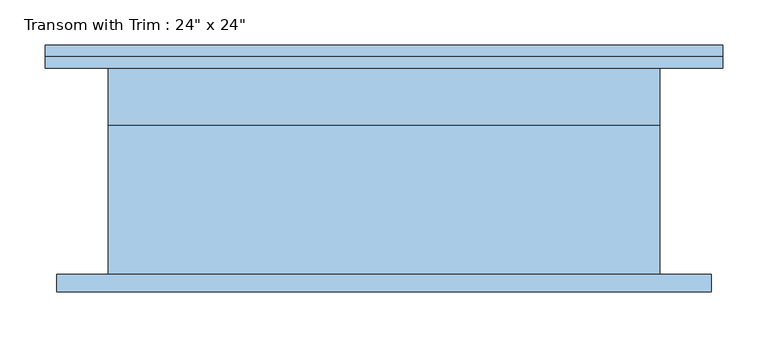
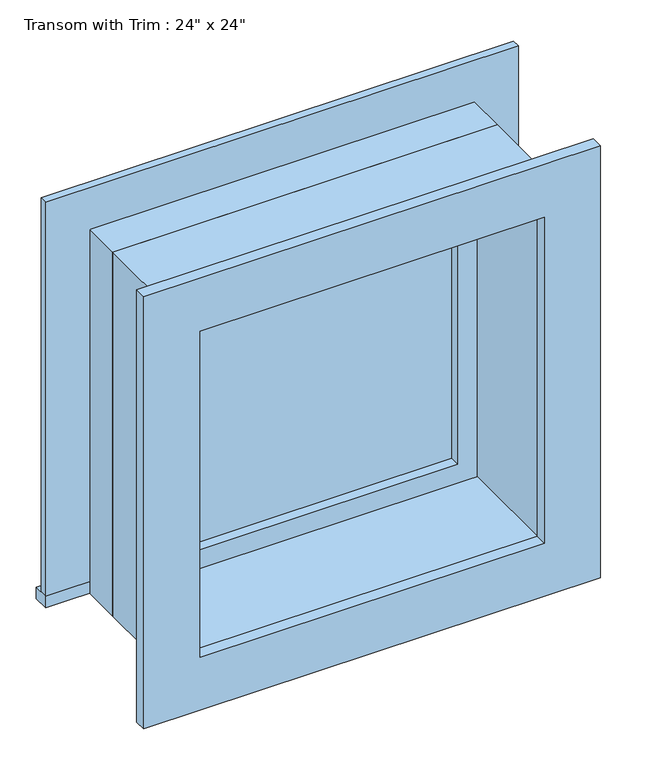
"""IFC4 building model written with IfcOpenShell, lengths in millimetres: window geometry."""

from ifc_helpers import new_model, si_unit, frame, origin, place, context, project, spatial, polyline, outline, extrude, source, transform, mapped, element, save


def window_3ed046d9(model_context):
    return source(origin(), model_context, "Body", "SweptSolid", [
        extrude(outline(polyline([(-412.75, 139.7), (336.55, 139.7), (336.55, 114.3), (-412.75, 114.3), (-412.75, 139.7)])), frame((0.0, 0.0, 2159.0), z_axis=(0.0, 0.0, 1.0), x_axis=(1.0, 0.0, 0.0)), (0.0, 0.0, 1.0), 19.05),
        extrude(outline(polyline([(2749.55, -323.85), (2749.55, 247.65), (2178.05, 247.65), (2178.05, 336.55), (2838.45, 336.55), (2838.45, -412.75), (2178.05, -412.75), (2178.05, -323.85), (2749.55, -323.85)])), frame((0.0, 114.3, 0.0), z_axis=(0.0, 1.0, 0.0), x_axis=(0.0, 0.0, 1.0)), (0.0, 0.0, 1.0), 12.7),
        extrude(outline(polyline([(2825.75, 323.85), (2825.75, -400.05), (2101.85, -400.05), (2101.85, 323.85), (2825.75, 323.85)]), holes=[polyline([(2736.85, 234.95), (2190.75, 234.95), (2190.75, -311.15), (2736.85, -311.15), (2736.85, 234.95)])]), frame((0.0, -133.35, 0.0), z_axis=(0.0, 1.0, 0.0), x_axis=(0.0, 0.0, 1.0)), (0.0, 0.0, 1.0), 19.05),
        extrude(outline(polyline([(203.2, 66.675), (-279.4, 66.675), (-279.4, 79.375), (203.2, 79.375), (203.2, 66.675)])), frame((0.0, 0.0, 2222.5), z_axis=(0.0, 0.0, 1.0), x_axis=(1.0, 0.0, 0.0)), (0.0, 0.0, 1.0), 482.6),
        extrude(outline(polyline([(2749.55, -323.85), (2178.05, -323.85), (2178.05, 247.65), (2749.55, 247.65), (2749.55, -323.85)]), holes=[polyline([(2705.1, -279.4), (2705.1, 203.2), (2222.5, 203.2), (2222.5, -279.4), (2705.1, -279.4)])]), frame((0.0, 50.8, 0.0), z_axis=(0.0, 1.0, 0.0), x_axis=(0.0, 0.0, 1.0)), (0.0, 0.0, 1.0), 44.45),
        extrude(outline(polyline([(2768.6, -342.9), (2159.0, -342.9), (2159.0, 266.7), (2768.6, 266.7), (2768.6, -342.9)]), holes=[polyline([(2736.85, -311.15), (2736.85, 234.95), (2190.75, 234.95), (2190.75, -311.15), (2736.85, -311.15)])]), frame((0.0, -114.3, 0.0), z_axis=(0.0, 1.0, 0.0), x_axis=(0.0, 0.0, 1.0)), (0.0, 0.0, 1.0), 165.1),
        extrude(outline(polyline([(2768.6, 266.7), (2768.6, -342.9), (2159.0, -342.9), (2159.0, 266.7), (2768.6, 266.7)]), holes=[polyline([(2749.55, 247.65), (2178.05, 247.65), (2178.05, -323.85), (2749.55, -323.85), (2749.55, 247.65)])]), frame((0.0, 50.8, 0.0), z_axis=(0.0, 1.0, 0.0), x_axis=(0.0, 0.0, 1.0)), (0.0, 0.0, 1.0), 63.5),
    ])


if __name__ == "__main__":
    model = new_model("IFC4")
    model_context = context("Model", 3, world=origin())
    ifc_project = project(units=[si_unit("LENGTHUNIT", "METRE", prefix="MILLI")], contexts=[model_context])
    site = spatial("IfcSite", under=ifc_project)
    building = spatial("IfcBuilding", under=site)
    placement = place(None, origin())
    window_shape = window_3ed046d9(model_context)
    element("IfcWindow", 1, ObjectType="Transom with Trim : 24\" x 24\"", at=placement, inside=building, context=model_context, shape_type="MappedRepresentation", body=[
        mapped(window_shape, transform((0.0, 0.0, 0.0), x_axis=(1.0, 0.0, 0.0), y_axis=(0.0, 1.0, 0.0), z_axis=(0.0, 0.0, 1.0))),
    ])
    save(model, "model.ifc")

# Revit data of these elements
# Type "Transom with Trim : 24\" x 24\""
#   Type Mark = "20"
#   Construction Type Id = "GSP4R"
#   Assembly Code = "B2020100"
#   Analytic Construction = "1/8 in Pilkington single glazing"
#   Visual Light Transmittance = 0.9
#   Solar Heat Gain Coefficient = 0.78
#   Heat Transfer Coefficient (U) = 0.6496 BTU/(h·ft²·°F)
#   Height = 2' - 0"
#   Default Sill Height = 7' - 1"
#   Trim Projection - Ext. = 0' - 0 1/2"
#   Trim Projection - Int. = 0' - 0 3/4"
#   Trim Width - Exterior = 0' - 3 1/2"
#   Trim Width - Interior = 0' - 3 1/2"
#   Width = 2' - 0"
#   Window Inset = 0' - 0 3/4"
#   Define Thermal Properties by = 1
#   Glass Pane Material = Glass
#   Sash Material = Sash
#   Trim Exterior Material = Trim
#   Trim Interior Material = Trim
#   Wall Closure = (empty or 0)
# Element 1 (IfcWindow, "Transom with Trim : 24\" x 24\"")
#   Materials on its faces: "Sash", "Trim", "Glass"
# Materials
#   "Glass": class "Glass", colour RGB 0 128 192, transparency 0.75, Description = "Soda Lime Glass", Cost = 0
#   "Sash": class "Wood", colour RGB 224 178 126, transparency 0
#   "Trim": class "Wood", colour RGB 224 178 126, transparency 0
